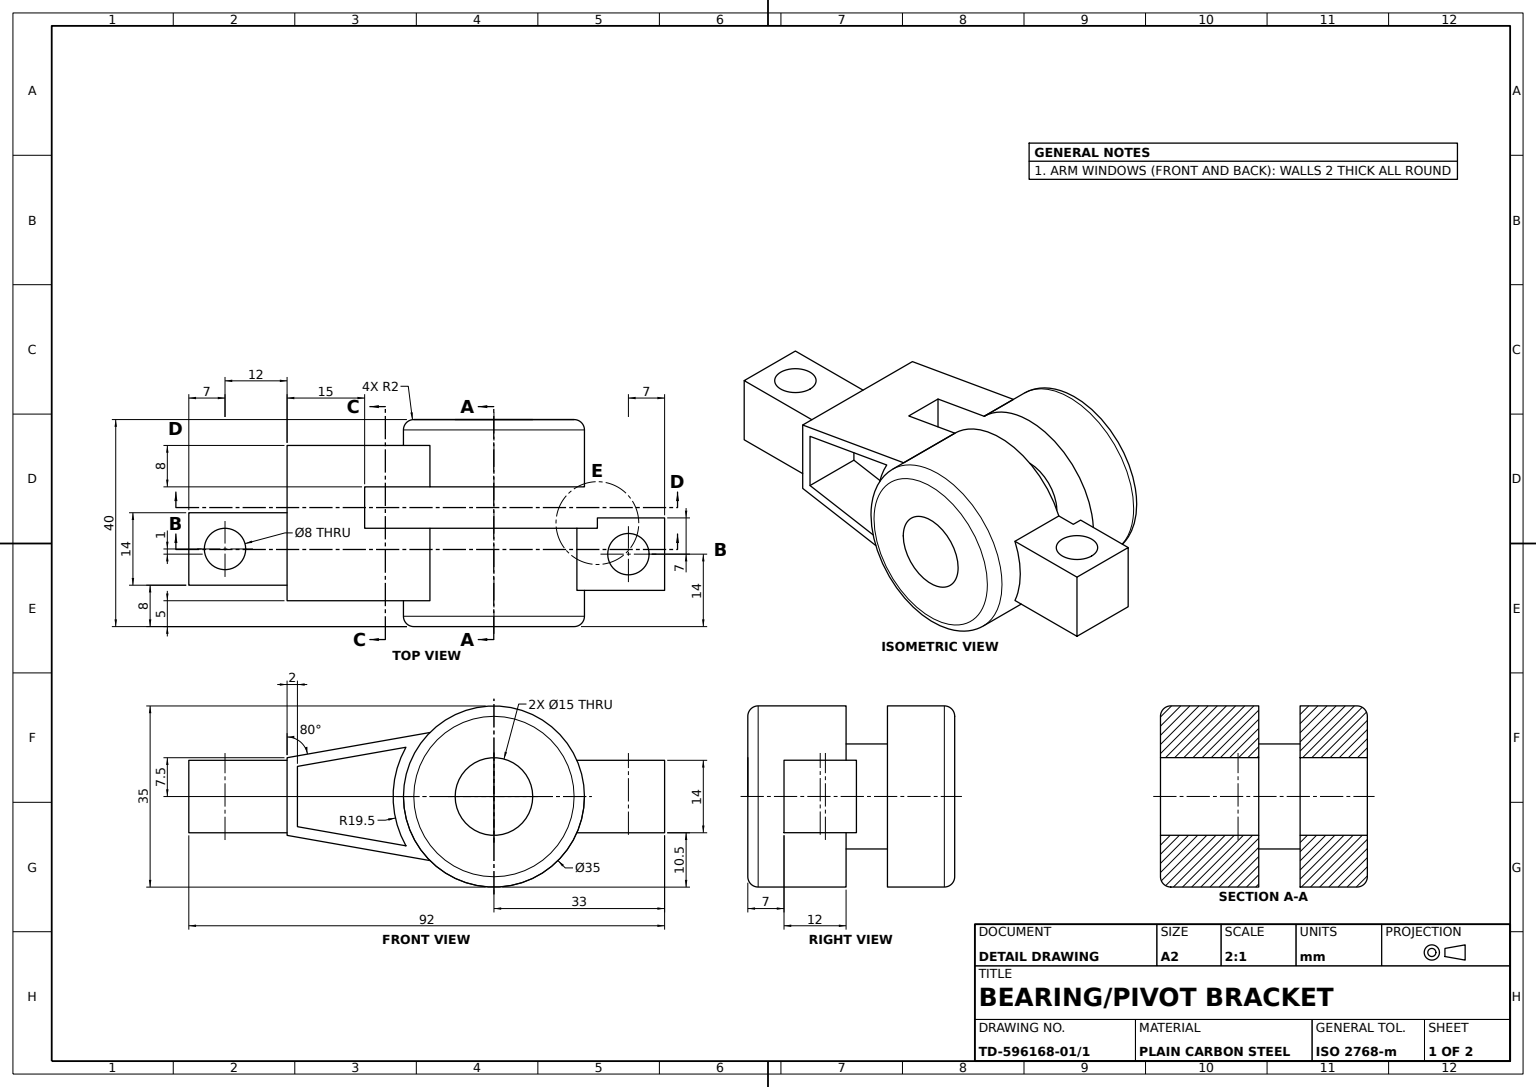
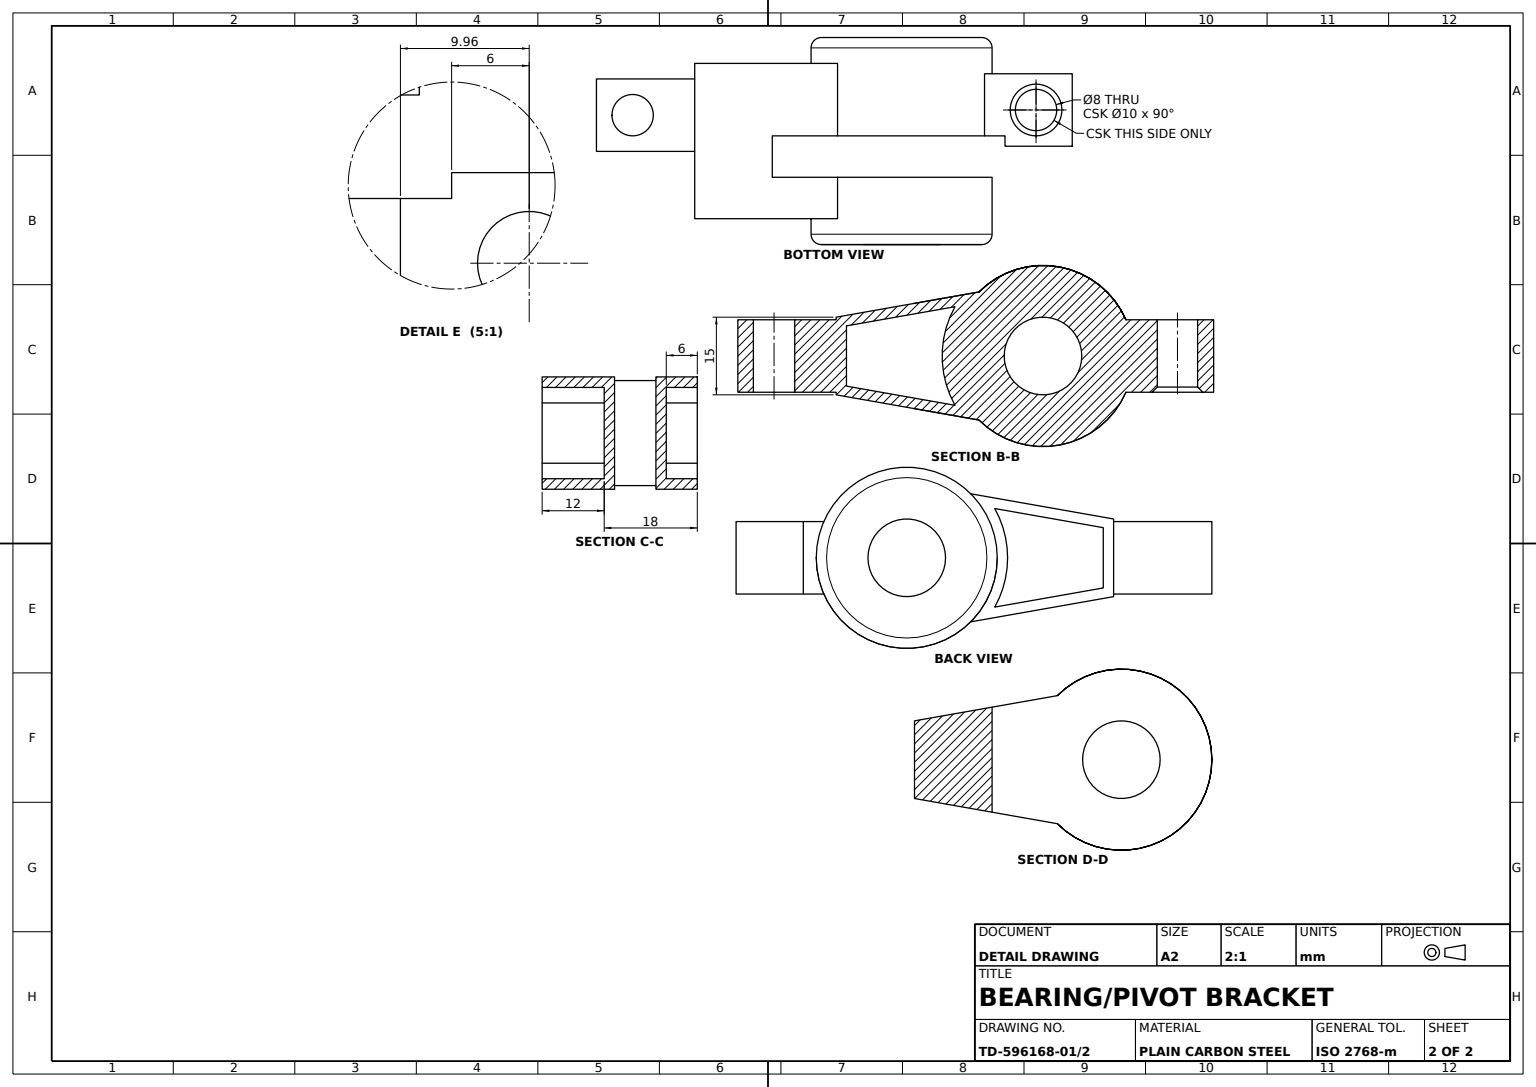
from build123d import *
from build123d.topology import SkipClean

# Parameters (mm, degrees)
BRACKET_SIDE_PROFILE_SKETCH_R = 7.5
BRACKET_BODY_40MM_DEPTH       = 20
TOP_SLOT_CUT_15X19_DEPTH      = 54.124852941
TOP_SLOT_CUT_15X19_DEPTH_BACK = 54.124852941
TOP_SLOT_SKETCH_W             = 45
TOP_SLOT_SKETCH_H             = 8
SIDE_RELIEF_A_CUT_7MM_DEPTH   = 7
SIDE_RELIEF_B_SKETCH_W        = 19
SIDE_RELIEF_B_SKETCH_H        = 14
SIDE_RELIEF_B_CUT_7MM_DEPTH   = 7
LUG_TRIM_A_CUT_5MM_DEPTH      = 5
LUG_START                     = -5
LUG_TRIM_B_CUT_5MM_DEPTH      = 5
HUB_GAP_SKETCH_W              = 19
HUB_GAP_SKETCH_H              = 14
HUB_GAP_CUT_18MM_DEPTH        = 18
RELIEF_STEP_SKETCH_W          = 19
RELIEF_STEP_SKETCH_H          = 14
RELIEF_STEP_CUT_1MM_DEPTH     = 1
WINDOW_START                  = -19
WINDOW_OPENING_CUT_19MM_DEPTH = 19
LUG_HOLE_A_CUT_12MM_DEPTH     = 12
LUG_START_2                   = -6
LUG_HOLE_B_CUT_6MM_DEPTH      = 6
EDGE_FILLET_R2_R              = 2
HUB_BORE_CUT_REACH            = 57.823
HUB_BORE_SKETCH_R             = 4
BORE_CHAMFER_1X45_SIZE        = 1


with BuildPart() as part:
    # Bracket Side Profile Sketch → Bracket Body 40mm (new, symmetric)
    with BuildSketch(Plane.XY):
        with BuildLine():
            Line((-46, -7), (-46, 7))
            Line((-46, 7), (-27, 7))
            Line((-27, 7), (-27, 7.5))
            Line((-27, 7.5), (0.62171804, 12.370454144))
            ThreePointArc((0.62171804, 12.370454144), (16.249720896, 17.195619038), (29.039014932, 7))
            Line((29.039014932, 7), (46, 7))
            Line((46, 7), (46, -7))
            Line((46, -7), (29.039014932, -7))
            ThreePointArc((29.039014932, -7), (16.249720896, -17.195619038), (0.62171804, -12.370454144))
            Line((0.62171804, -12.370454144), (-27, -7.5))
            Line((-27, -7.5), (-27, -7))
            Line((-27, -7), (-46, -7))
        make_face()
        with Locations((13, 0)):
            Circle(BRACKET_SIDE_PROFILE_SKETCH_R, mode=Mode.SUBTRACT)
    extrude(amount=BRACKET_BODY_40MM_DEPTH, both=True)

    # Top Slot Sketch → Top Slot Cut 15x19 (cut, two sides: drawn at the far end of the back side and taken through both)
    with BuildSketch(Plane(origin=(0, 0, 0), x_dir=(1, 0, 0), z_dir=(0, 1, 0)).offset(-TOP_SLOT_CUT_15X19_DEPTH_BACK)):
        with Locations((10.5, 3)):
            Rectangle(TOP_SLOT_SKETCH_W, TOP_SLOT_SKETCH_H)
    extrude(amount=TOP_SLOT_CUT_15X19_DEPTH + TOP_SLOT_CUT_15X19_DEPTH_BACK, mode=Mode.SUBTRACT)

    # Side Relief A Sketch → Side Relief A Cut 7mm (cut)
    with BuildSketch(Plane.XY.offset(20)):
        with BuildLine():
            Line((29.039014932, -7), (46, -7))
            Line((46, -7), (46, 7))
            Line((46, 7), (29.039014932, 7))
            ThreePointArc((29.039014932, 7), (30.5, 0), (29.039014932, -7))
        make_face()
    extrude(amount=-SIDE_RELIEF_A_CUT_7MM_DEPTH, mode=Mode.SUBTRACT)

    # Side Relief B Sketch → Side Relief B Cut 7mm (cut)
    with BuildSketch(Plane.XY.offset(20)):
        with Locations((-36.5, 0)):
            Rectangle(SIDE_RELIEF_B_SKETCH_W, SIDE_RELIEF_B_SKETCH_H)
    extrude(amount=-SIDE_RELIEF_B_CUT_7MM_DEPTH, mode=Mode.SUBTRACT)

    # Lug Trim A Sketch → Lug Trim A Cut 5mm (cut)
    with SkipClean():  # the faces are left unmerged after this step: merging them gives an invalid solid
        with BuildSketch(Plane.XY.offset(20)):
            with BuildLine():
                ThreePointArc((0.62171804, 12.370454144), (-4.5, 0), (0.62171804, -12.370454144))
                Line((0.62171804, -12.370454144), (-27, -7.5))
                Line((-27, -7.5), (-27, 7.5))
                Line((-27, 7.5), (0.62171804, 12.370454144))
            make_face()
        extrude(amount=-LUG_TRIM_A_CUT_5MM_DEPTH, mode=Mode.SUBTRACT)

    # Lug Trim B Sketch → Lug Trim B Cut 5mm (cut)
    with SkipClean():  # the faces are left unmerged after this step: merging them gives an invalid solid
        with BuildSketch(Plane(origin=(0, 0, -20), x_dir=(-1, 0, 0), z_dir=(0, 0, -1)).offset(LUG_START)):
            with BuildLine():
                Line((27, -7.5), (-0.62171804, -12.370454144))
                ThreePointArc((-0.62171804, -12.370454144), (4.5, 0), (-0.62171804, 12.370454144))
                Line((-0.62171804, 12.370454144), (27, 7.5))
                Line((27, 7.5), (27, -7.5))
            make_face()
        extrude(amount=LUG_TRIM_B_CUT_5MM_DEPTH, mode=Mode.SUBTRACT)

    # Hub Gap Sketch → Hub Gap Cut 18mm (cut)
    with SkipClean():  # the faces are left unmerged after this step: merging them gives an invalid solid
        with BuildSketch(Plane(origin=(0, 0, -20), x_dir=(-1, 0, 0), z_dir=(0, 0, -1))):
            with Locations((36.5, 0)):
                Rectangle(HUB_GAP_SKETCH_W, HUB_GAP_SKETCH_H)
        extrude(amount=-HUB_GAP_CUT_18MM_DEPTH, mode=Mode.SUBTRACT)

    # Relief Step Sketch → Relief Step Cut 1mm (cut)
    with SkipClean():  # the faces are left unmerged after this step: merging them gives an invalid solid
        with BuildSketch(Plane.XY.offset(13)):
            with Locations((-36.5, 0)):
                Rectangle(RELIEF_STEP_SKETCH_W, RELIEF_STEP_SKETCH_H)
        extrude(amount=-RELIEF_STEP_CUT_1MM_DEPTH, mode=Mode.SUBTRACT)

    # Window Opening Sketch → Window Opening Cut 19mm (cut)
    with SkipClean():  # the faces are left unmerged after this step: merging them gives an invalid solid
        with BuildSketch(Plane(origin=(0, 0, -20), x_dir=(-1, 0, 0), z_dir=(0, 0, -1)).offset(WINDOW_START)):
            with BuildLine():
                Line((-29.039014932, 7), (-46, 7))
                Line((-46, 7), (-46, -7))
                Line((-46, -7), (-29.039014932, -7))
                ThreePointArc((-29.039014932, -7), (-30.5, 0), (-29.039014932, 7))
            make_face()
        extrude(amount=WINDOW_OPENING_CUT_19MM_DEPTH, mode=Mode.SUBTRACT)

    # Lug Hole A Sketch → Lug Hole A Cut 12mm (cut)
    with SkipClean():  # the faces are left unmerged after this step: merging them gives an invalid solid
        with BuildSketch(Plane.XY.offset(15)):
            with BuildLine():
                Line((-4.017310196, 9.521615078), (-25, 5.821800738))
                Line((-25, 5.821800738), (-25, -5.821800738))
                Line((-25, -5.821800738), (-4.017310196, -9.521615078))
                ThreePointArc((-4.017310196, -9.521615078), (-6.5, 0), (-4.017310196, 9.521615078))
            make_face()
        extrude(amount=-LUG_HOLE_A_CUT_12MM_DEPTH, mode=Mode.SUBTRACT)

    # Lug Hole B Sketch → Lug Hole B Cut 6mm (cut)
    with SkipClean():  # the faces are left unmerged after this step: merging them gives an invalid solid
        with BuildSketch(Plane(origin=(0, 0, -15), x_dir=(-1, 0, 0), z_dir=(0, 0, -1)).offset(LUG_START_2)):
            with BuildLine():
                Line((4.017310196, -9.521615078), (25, -5.821800738))
                Line((25, -5.821800738), (25, 5.821800738))
                Line((25, 5.821800738), (4.017310196, 9.521615078))
                ThreePointArc((4.017310196, 9.521615078), (6.5, 0), (4.017310196, -9.521615078))
            make_face()
        extrude(amount=LUG_HOLE_B_CUT_6MM_DEPTH, mode=Mode.SUBTRACT)

    # Edge Fillet R2
    edge_fillet_r2_edges = [part.edges().sort_by_distance(p)[0] for p in [
        (30.5, 0, -20),
        (30.5, 0, 20),
    ]]
    fillet(edge_fillet_r2_edges, radius=EDGE_FILLET_R2_R)

    # Hub Bore Sketch → Hub Bore Cut (cut, up to next)
    with BuildSketch(Plane(origin=(0, 7, 0), x_dir=(1, 0, 0), z_dir=(0, 1, 0)), mode=Mode.PRIVATE) as hub_bore_cut_sk1:
        with Locations(Location((-39, -5, 0), (0, 0, 180))):
            Circle(HUB_BORE_SKETCH_R)
    hub_bore_cut_tool1 = extrude(hub_bore_cut_sk1.sketch, amount=-HUB_BORE_CUT_REACH, mode=Mode.PRIVATE) & part.part
    # Hub Bore Sketch → Hub Bore Cut (cut, up to next)
    with BuildSketch(Plane(origin=(0, 7, 0), x_dir=(1, 0, 0), z_dir=(0, 1, 0)), mode=Mode.PRIVATE) as hub_bore_cut_sk2:
        with Locations(Location((39, -6, 0), (0, 0, 180))):
            Circle(HUB_BORE_SKETCH_R)
    hub_bore_cut_tool2 = extrude(hub_bore_cut_sk2.sketch, amount=-HUB_BORE_CUT_REACH, mode=Mode.PRIVATE) & part.part
    add(hub_bore_cut_tool1.solids().sort_by_distance((-39, 7, 5))[0], mode=Mode.SUBTRACT)
    add(hub_bore_cut_tool2.solids().sort_by_distance((39, 7, 6))[0], mode=Mode.SUBTRACT)

    # Bore Chamfer 1x45
    bore_chamfer_1x45_edges = [part.edges().sort_by_distance(p)[0] for p in [
        (43, -7, 6),
    ]]
    chamfer(bore_chamfer_1x45_edges, length=BORE_CHAMFER_1X45_SIZE)


solid = part.part
